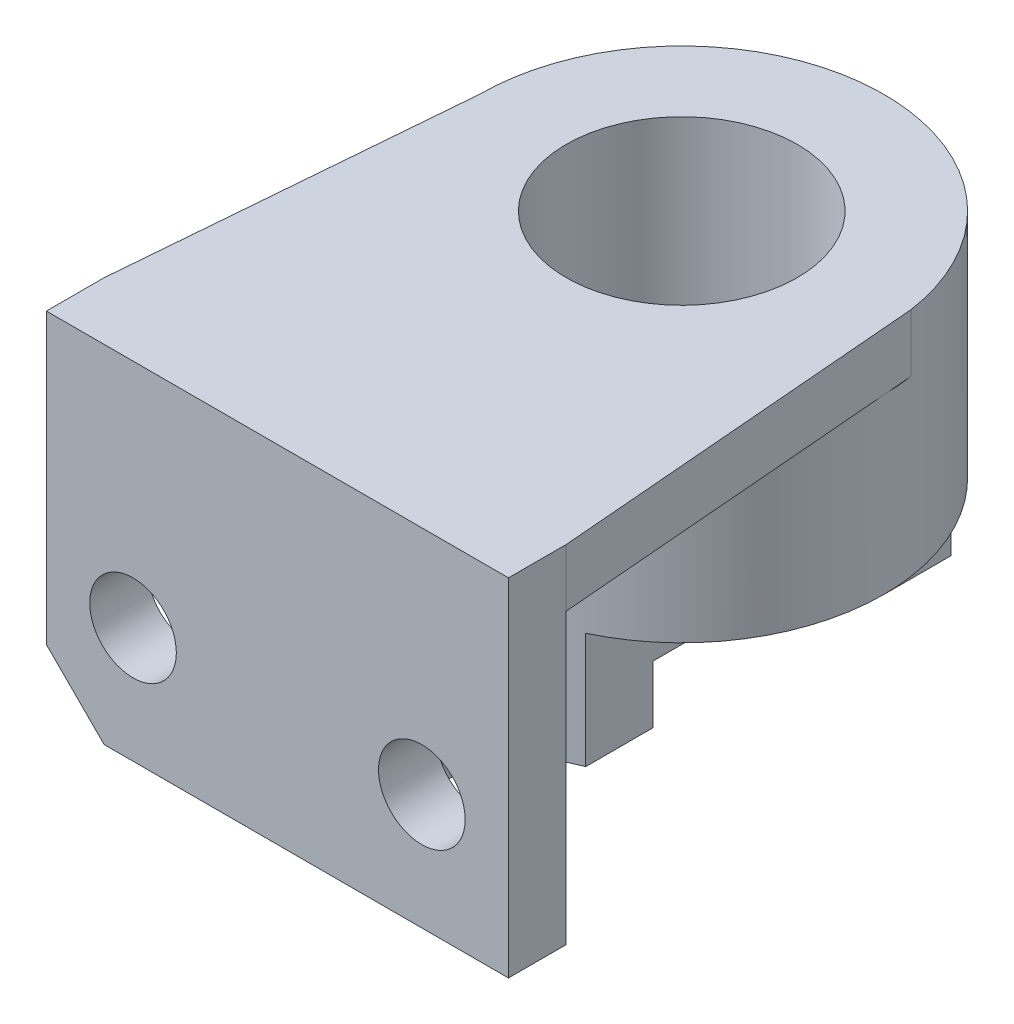
ISO-10303-21;
HEADER;
FILE_DESCRIPTION(('STEP AP214'),'2;1');
FILE_NAME('part.step','',(''),(''),'','','');
FILE_SCHEMA(('AUTOMOTIVE_DESIGN { 1 0 10303 214 1 1 1 1 }'));
ENDSEC;
DATA;
#1=APPLICATION_CONTEXT('core data for automotive mechanical design processes');
#2=APPLICATION_PROTOCOL_DEFINITION('international standard','automotive_design',2000,#1);
#3=PRODUCT_CONTEXT('',#1,'mechanical');
#4=PRODUCT('Part','Part','',(#3));
#5=PRODUCT_RELATED_PRODUCT_CATEGORY('part','',(#4));
#6=PRODUCT_DEFINITION_FORMATION('','',#4);
#7=PRODUCT_DEFINITION_CONTEXT('part definition',#1,'design');
#8=PRODUCT_DEFINITION('design','',#6,#7);
#9=PRODUCT_DEFINITION_SHAPE('','',#8);
#10=(LENGTH_UNIT() NAMED_UNIT(*) SI_UNIT(.MILLI.,.METRE.));
#11=(NAMED_UNIT(*) PLANE_ANGLE_UNIT() SI_UNIT($,.RADIAN.));
#12=(NAMED_UNIT(*) SI_UNIT($,.STERADIAN.) SOLID_ANGLE_UNIT());
#13=UNCERTAINTY_MEASURE_WITH_UNIT(LENGTH_MEASURE(1.E-05),#10,'distance_accuracy_value','');
#14=(GEOMETRIC_REPRESENTATION_CONTEXT(3) GLOBAL_UNCERTAINTY_ASSIGNED_CONTEXT((#13)) GLOBAL_UNIT_ASSIGNED_CONTEXT((#10,
#11,#12)) REPRESENTATION_CONTEXT('',''));
#15=CARTESIAN_POINT('',(0.,0.,0.));
#16=DIRECTION('',(0.,0.,1.));
#17=DIRECTION('',(1.,0.,0.));
#18=AXIS2_PLACEMENT_3D('',#15,#16,#17);
#19=CARTESIAN_POINT('',(40.,10.,-60.));
#20=DIRECTION('',(0.,-1.,0.));
#21=DIRECTION('',(0.,0.,-1.));
#22=AXIS2_PLACEMENT_3D('',#19,#20,#21);
#23=PLANE('',#22);
#24=CARTESIAN_POINT('',(40.,10.,-60.));
#25=DIRECTION('',(0.,-1.,0.));
#26=DIRECTION('',(0.,0.,-1.));
#27=AXIS2_PLACEMENT_3D('',#24,#25,#26);
#28=CIRCLE('',#27,20.);
#29=CARTESIAN_POINT('',(55.,10.,-73.228756555323));
#30=VERTEX_POINT('',#29);
#31=CARTESIAN_POINT('',(55.,10.,-46.771243444677));
#32=VERTEX_POINT('',#31);
#33=EDGE_CURVE('E213',#30,#32,#28,.T.);
#34=ORIENTED_EDGE('',*,*,#33,.F.);
#35=DIRECTION('',(0.,0.,-1.));
#36=VECTOR('',#35,1.);
#37=CARTESIAN_POINT('',(55.,10.,-28.3772233983162));
#38=LINE('',#37,#36);
#39=CARTESIAN_POINT('',(55.,10.,-91.6227766016838));
#40=VERTEX_POINT('',#39);
#41=EDGE_CURVE('E212',#30,#40,#38,.T.);
#42=ORIENTED_EDGE('',*,*,#41,.T.);
#43=CARTESIAN_POINT('',(40.,10.,-60.));
#44=DIRECTION('',(0.,-1.,0.));
#45=DIRECTION('',(0.,0.,-1.));
#46=AXIS2_PLACEMENT_3D('',#43,#44,#45);
#47=CIRCLE('',#46,35.);
#48=CARTESIAN_POINT('',(55.,10.,-28.3772233983162));
#49=VERTEX_POINT('',#48);
#50=EDGE_CURVE('E230',#40,#49,#47,.T.);
#51=ORIENTED_EDGE('',*,*,#50,.T.);
#52=EDGE_CURVE('E217',#49,#32,#38,.T.);
#53=ORIENTED_EDGE('',*,*,#52,.T.);
#54=EDGE_LOOP('',(#34,#42,#51,#53));
#55=FACE_BOUND('',#54,.T.);
#56=ADVANCED_FACE('F50',(#55),#23,.T.);
#57=CARTESIAN_POINT('',(40.,-10.,-60.));
#58=DIRECTION('',(0.,-1.,0.));
#59=DIRECTION('',(0.,0.,-1.));
#60=AXIS2_PLACEMENT_3D('',#57,#58,#59);
#61=PLANE('',#60);
#62=DIRECTION('',(0.,0.,-1.));
#63=VECTOR('',#62,1.);
#64=CARTESIAN_POINT('',(55.,-10.,-28.3772233983162));
#65=LINE('',#64,#63);
#66=CARTESIAN_POINT('',(55.,-10.,-28.3772233983162));
#67=VERTEX_POINT('',#66);
#68=CARTESIAN_POINT('',(55.,-10.,-40.));
#69=VERTEX_POINT('',#68);
#70=EDGE_CURVE('E445',#67,#69,#65,.T.);
#71=ORIENTED_EDGE('',*,*,#70,.F.);
#72=CARTESIAN_POINT('',(40.,-10.,-60.));
#73=DIRECTION('',(0.,-1.,0.));
#74=DIRECTION('',(0.,0.,-1.));
#75=AXIS2_PLACEMENT_3D('',#72,#73,#74);
#76=CIRCLE('',#75,35.);
#77=CARTESIAN_POINT('',(45.0000000000001,-10.,-25.3589838486225));
#78=VERTEX_POINT('',#77);
#79=EDGE_CURVE('E311',#67,#78,#76,.T.);
#80=ORIENTED_EDGE('',*,*,#79,.T.);
#81=DIRECTION('',(0.,0.,1.));
#82=VECTOR('',#81,1.);
#83=CARTESIAN_POINT('',(45.0000000000001,-10.,-25.3589838486225));
#84=LINE('',#83,#82);
#85=CARTESIAN_POINT('',(45.,-10.,0.));
#86=VERTEX_POINT('',#85);
#87=EDGE_CURVE('E288',#78,#86,#84,.T.);
#88=ORIENTED_EDGE('',*,*,#87,.T.);
#89=DIRECTION('',(1.,0.,0.));
#90=VECTOR('',#89,1.);
#91=CARTESIAN_POINT('',(0.,-10.,0.));
#92=LINE('',#91,#90);
#93=CARTESIAN_POINT('',(80.,-10.,0.));
#94=VERTEX_POINT('',#93);
#95=EDGE_CURVE('E282',#86,#94,#92,.T.);
#96=ORIENTED_EDGE('',*,*,#95,.T.);
#97=DIRECTION('',(0.,0.,1.));
#98=VECTOR('',#97,1.);
#99=CARTESIAN_POINT('',(80.,-10.,0.));
#100=LINE('',#99,#98);
#101=CARTESIAN_POINT('',(80.,-10.,10.));
#102=VERTEX_POINT('',#101);
#103=EDGE_CURVE('E276',#94,#102,#100,.T.);
#104=ORIENTED_EDGE('',*,*,#103,.T.);
#105=DIRECTION('',(1.,0.,0.));
#106=VECTOR('',#105,1.);
#107=CARTESIAN_POINT('',(0.,-10.,10.));
#108=LINE('',#107,#106);
#109=CARTESIAN_POINT('',(10.,-10.,10.));
#110=VERTEX_POINT('',#109);
#111=EDGE_CURVE('E278',#110,#102,#108,.T.);
#112=ORIENTED_EDGE('',*,*,#111,.F.);
#113=DIRECTION('',(0.,0.,1.));
#114=VECTOR('',#113,1.);
#115=CARTESIAN_POINT('',(10.,-10.,0.));
#116=LINE('',#115,#114);
#117=CARTESIAN_POINT('',(9.99999999999999,-10.,0.));
#118=VERTEX_POINT('',#117);
#119=EDGE_CURVE('E272',#118,#110,#116,.T.);
#120=ORIENTED_EDGE('',*,*,#119,.F.);
#121=CARTESIAN_POINT('',(35.,-10.,0.));
#122=VERTEX_POINT('',#121);
#123=EDGE_CURVE('E277',#118,#122,#92,.T.);
#124=ORIENTED_EDGE('',*,*,#123,.T.);
#125=DIRECTION('',(0.,0.,-1.));
#126=VECTOR('',#125,1.);
#127=CARTESIAN_POINT('',(35.,-10.,0.));
#128=LINE('',#127,#126);
#129=CARTESIAN_POINT('',(35.,-10.,-25.3589838486225));
#130=VERTEX_POINT('',#129);
#131=EDGE_CURVE('E283',#122,#130,#128,.T.);
#132=ORIENTED_EDGE('',*,*,#131,.T.);
#133=CARTESIAN_POINT('',(25.,-10.,-28.3772233983162));
#134=VERTEX_POINT('',#133);
#135=EDGE_CURVE('E306',#130,#134,#76,.T.);
#136=ORIENTED_EDGE('',*,*,#135,.T.);
#137=DIRECTION('',(0.,0.,1.));
#138=VECTOR('',#137,1.);
#139=CARTESIAN_POINT('',(25.,-10.,-91.6227766016838));
#140=LINE('',#139,#138);
#141=CARTESIAN_POINT('',(25.,-10.,-40.));
#142=VERTEX_POINT('',#141);
#143=EDGE_CURVE('E426',#142,#134,#140,.T.);
#144=ORIENTED_EDGE('',*,*,#143,.F.);
#145=CARTESIAN_POINT('',(40.,-10.,-60.));
#146=DIRECTION('',(0.,-1.,0.));
#147=DIRECTION('',(0.,0.,-1.));
#148=AXIS2_PLACEMENT_3D('',#145,#146,#147);
#149=CIRCLE('',#148,25.);
#150=EDGE_CURVE('E254',#69,#142,#149,.T.);
#151=ORIENTED_EDGE('',*,*,#150,.F.);
#152=EDGE_LOOP('',(#71,#80,#88,#96,#104,#112,#120,#124,#132,#136,#144,#151));
#153=FACE_BOUND('',#152,.T.);
#154=ADVANCED_FACE('F397',(#153),#61,.T.);
#155=CARTESIAN_POINT('',(40.,0.,-60.));
#156=DIRECTION('',(0.,-1.,0.));
#157=DIRECTION('',(0.,0.,-1.));
#158=AXIS2_PLACEMENT_3D('',#155,#156,#157);
#159=CYLINDRICAL_SURFACE('',#158,25.);
#160=CARTESIAN_POINT('',(25.,-10.,-80.));
#161=VERTEX_POINT('',#160);
#162=CARTESIAN_POINT('',(55.,-10.,-80.));
#163=VERTEX_POINT('',#162);
#164=EDGE_CURVE('E251',#161,#163,#149,.T.);
#165=ORIENTED_EDGE('',*,*,#164,.T.);
#166=DIRECTION('',(0.,-1.,0.));
#167=VECTOR('',#166,1.);
#168=CARTESIAN_POINT('',(55.,0.,-80.));
#169=LINE('',#168,#167);
#170=CARTESIAN_POINT('',(55.,0.,-80.));
#171=VERTEX_POINT('',#170);
#172=EDGE_CURVE('E237',#163,#171,#169,.F.);
#173=ORIENTED_EDGE('',*,*,#172,.T.);
#174=CARTESIAN_POINT('',(40.,0.,-60.));
#175=DIRECTION('',(0.,-1.,0.));
#176=DIRECTION('',(0.,0.,-1.));
#177=AXIS2_PLACEMENT_3D('',#174,#175,#176);
#178=CIRCLE('',#177,25.);
#179=CARTESIAN_POINT('',(25.,0.,-80.));
#180=VERTEX_POINT('',#179);
#181=EDGE_CURVE('E248',#180,#171,#178,.T.);
#182=ORIENTED_EDGE('',*,*,#181,.F.);
#183=DIRECTION('',(0.,-1.,0.));
#184=VECTOR('',#183,1.);
#185=CARTESIAN_POINT('',(25.,0.,-80.));
#186=LINE('',#185,#184);
#187=EDGE_CURVE('E451',#180,#161,#186,.T.);
#188=ORIENTED_EDGE('',*,*,#187,.T.);
#189=EDGE_LOOP('',(#165,#173,#182,#188));
#190=FACE_BOUND('',#189,.T.);
#191=ADVANCED_FACE('F496',(#190),#159,.F.);
#192=CARTESIAN_POINT('',(40.,0.,-60.));
#193=DIRECTION('',(0.,-1.,0.));
#194=DIRECTION('',(0.,0.,-1.));
#195=AXIS2_PLACEMENT_3D('',#192,#193,#194);
#196=PLANE('',#195);
#197=DIRECTION('',(0.,0.,-1.));
#198=VECTOR('',#197,1.);
#199=CARTESIAN_POINT('',(55.,0.,-60.));
#200=LINE('',#199,#198);
#201=CARTESIAN_POINT('',(55.,0.,-40.));
#202=VERTEX_POINT('',#201);
#203=CARTESIAN_POINT('',(55.,0.,-46.771243444677));
#204=VERTEX_POINT('',#203);
#205=EDGE_CURVE('E241',#202,#204,#200,.T.);
#206=ORIENTED_EDGE('',*,*,#205,.F.);
#207=CARTESIAN_POINT('',(25.,0.,-40.));
#208=VERTEX_POINT('',#207);
#209=EDGE_CURVE('E255',#202,#208,#178,.T.);
#210=ORIENTED_EDGE('',*,*,#209,.T.);
#211=DIRECTION('',(0.,0.,1.));
#212=VECTOR('',#211,1.);
#213=CARTESIAN_POINT('',(25.,0.,-60.));
#214=LINE('',#213,#212);
#215=CARTESIAN_POINT('',(25.,0.,-46.7712434446771));
#216=VERTEX_POINT('',#215);
#217=EDGE_CURVE('E454',#216,#208,#214,.T.);
#218=ORIENTED_EDGE('',*,*,#217,.F.);
#219=CARTESIAN_POINT('',(40.,0.,-60.));
#220=DIRECTION('',(0.,-1.,0.));
#221=DIRECTION('',(0.,0.,-1.));
#222=AXIS2_PLACEMENT_3D('',#219,#220,#221);
#223=CIRCLE('',#222,20.);
#224=EDGE_CURVE('E247',#204,#216,#223,.T.);
#225=ORIENTED_EDGE('',*,*,#224,.F.);
#226=EDGE_LOOP('',(#206,#210,#218,#225));
#227=FACE_BOUND('',#226,.T.);
#228=ADVANCED_FACE('F444',(#227),#196,.T.);
#229=CARTESIAN_POINT('',(0.,0.,0.));
#230=DIRECTION('',(0.,0.,1.));
#231=DIRECTION('',(1.,0.,0.));
#232=AXIS2_PLACEMENT_3D('',#229,#230,#231);
#233=PLANE('',#232);
#234=CARTESIAN_POINT('',(65.,10.,0.));
#235=DIRECTION('',(0.,0.,1.));
#236=DIRECTION('',(1.,0.,0.));
#237=AXIS2_PLACEMENT_3D('',#234,#235,#236);
#238=CIRCLE('',#237,7.50000000000001);
#239=CARTESIAN_POINT('',(72.5,10.,0.));
#240=VERTEX_POINT('',#239);
#241=EDGE_CURVE('E261',#240,#240,#238,.T.);
#242=ORIENTED_EDGE('',*,*,#241,.T.);
#243=EDGE_LOOP('',(#242));
#244=FACE_BOUND('',#243,.T.);
#245=DIRECTION('',(0.,1.,0.));
#246=VECTOR('',#245,1.);
#247=CARTESIAN_POINT('',(80.,10.,0.));
#248=LINE('',#247,#246);
#249=CARTESIAN_POINT('',(80.,40.,0.));
#250=VERTEX_POINT('',#249);
#251=EDGE_CURVE('E345',#94,#250,#248,.T.);
#252=ORIENTED_EDGE('',*,*,#251,.F.);
#253=ORIENTED_EDGE('',*,*,#95,.F.);
#254=DIRECTION('',(0.,-1.,0.));
#255=VECTOR('',#254,1.);
#256=CARTESIAN_POINT('',(45.,40.,0.));
#257=LINE('',#256,#255);
#258=CARTESIAN_POINT('',(45.,40.,0.));
#259=VERTEX_POINT('',#258);
#260=EDGE_CURVE('E294',#259,#86,#257,.T.);
#261=ORIENTED_EDGE('',*,*,#260,.F.);
#262=DIRECTION('',(-1.,0.,0.));
#263=VECTOR('',#262,1.);
#264=CARTESIAN_POINT('',(0.,40.,0.));
#265=LINE('',#264,#263);
#266=EDGE_CURVE('E324',#250,#259,#265,.T.);
#267=ORIENTED_EDGE('',*,*,#266,.F.);
#268=EDGE_LOOP('',(#252,#253,#261,#267));
#269=FACE_BOUND('',#268,.T.);
#270=ADVANCED_FACE('F401',(#244,#269),#233,.F.);
#271=CARTESIAN_POINT('',(0.,40.,0.));
#272=DIRECTION('',(0.,1.,0.));
#273=DIRECTION('',(0.,0.,1.));
#274=AXIS2_PLACEMENT_3D('',#271,#272,#273);
#275=PLANE('',#274);
#276=ORIENTED_EDGE('',*,*,#266,.T.);
#277=DIRECTION('',(0.,0.,1.));
#278=VECTOR('',#277,1.);
#279=CARTESIAN_POINT('',(45.0000000000001,40.,-25.3589838486225));
#280=LINE('',#279,#278);
#281=CARTESIAN_POINT('',(45.0000000000001,40.,-25.3589838486225));
#282=VERTEX_POINT('',#281);
#283=EDGE_CURVE('E290',#282,#259,#280,.T.);
#284=ORIENTED_EDGE('',*,*,#283,.F.);
#285=CARTESIAN_POINT('',(40.,40.,-60.));
#286=DIRECTION('',(0.,1.,0.));
#287=DIRECTION('',(0.,0.,1.));
#288=AXIS2_PLACEMENT_3D('',#285,#286,#287);
#289=CIRCLE('',#288,35.);
#290=CARTESIAN_POINT('',(74.9933136553649,40.,-60.6841048291398));
#291=VERTEX_POINT('',#290);
#292=EDGE_CURVE('E11',#291,#282,#289,.F.);
#293=ORIENTED_EDGE('',*,*,#292,.F.);
#294=DIRECTION('',(-0.0822247076971217,0.,-0.996613815599665));
#295=VECTOR('',#294,1.);
#296=CARTESIAN_POINT('',(79.4591277955298,40.,-6.55570237396765));
#297=LINE('',#296,#295);
#298=EDGE_CURVE('E313',#250,#291,#297,.T.);
#299=ORIENTED_EDGE('',*,*,#298,.F.);
#300=EDGE_LOOP('',(#276,#284,#293,#299));
#301=FACE_BOUND('',#300,.T.);
#302=ADVANCED_FACE('F390',(#301),#275,.F.);
#303=CARTESIAN_POINT('',(15.,10.,0.));
#304=DIRECTION('',(0.,0.,1.));
#305=DIRECTION('',(1.,0.,0.));
#306=AXIS2_PLACEMENT_3D('',#303,#304,#305);
#307=CIRCLE('',#306,7.5);
#308=CARTESIAN_POINT('',(22.5,10.,0.));
#309=VERTEX_POINT('',#308);
#310=EDGE_CURVE('E259',#309,#309,#307,.T.);
#311=ORIENTED_EDGE('',*,*,#310,.T.);
#312=EDGE_LOOP('',(#311));
#313=FACE_BOUND('',#312,.T.);
#314=ORIENTED_EDGE('',*,*,#123,.F.);
#315=DIRECTION('',(-0.707106781186548,0.707106781186548,0.));
#316=VECTOR('',#315,1.);
#317=CARTESIAN_POINT('',(10.,-10.,0.));
#318=LINE('',#317,#316);
#319=CARTESIAN_POINT('',(0.,0.,0.));
#320=VERTEX_POINT('',#319);
#321=EDGE_CURVE('E68',#118,#320,#318,.T.);
#322=ORIENTED_EDGE('',*,*,#321,.T.);
#323=DIRECTION('',(0.,-1.,0.));
#324=VECTOR('',#323,1.);
#325=CARTESIAN_POINT('',(0.,50.,0.));
#326=LINE('',#325,#324);
#327=CARTESIAN_POINT('',(0.,40.,0.));
#328=VERTEX_POINT('',#327);
#329=EDGE_CURVE('E337',#328,#320,#326,.T.);
#330=ORIENTED_EDGE('',*,*,#329,.F.);
#331=CARTESIAN_POINT('',(35.,40.,0.));
#332=VERTEX_POINT('',#331);
#333=EDGE_CURVE('E323',#332,#328,#265,.T.);
#334=ORIENTED_EDGE('',*,*,#333,.F.);
#335=DIRECTION('',(0.,-1.,0.));
#336=VECTOR('',#335,1.);
#337=CARTESIAN_POINT('',(35.,40.,0.));
#338=LINE('',#337,#336);
#339=EDGE_CURVE('E293',#332,#122,#338,.T.);
#340=ORIENTED_EDGE('',*,*,#339,.T.);
#341=EDGE_LOOP('',(#314,#322,#330,#334,#340));
#342=FACE_BOUND('',#341,.T.);
#343=ADVANCED_FACE('F420',(#313,#342),#233,.F.);
#344=CARTESIAN_POINT('',(0.,50.,10.));
#345=DIRECTION('',(1.,0.,0.));
#346=DIRECTION('',(0.,0.,-1.));
#347=AXIS2_PLACEMENT_3D('',#344,#345,#346);
#348=PLANE('',#347);
#349=ORIENTED_EDGE('',*,*,#329,.T.);
#350=DIRECTION('',(0.,0.,1.));
#351=VECTOR('',#350,1.);
#352=CARTESIAN_POINT('',(0.,0.,0.));
#353=LINE('',#352,#351);
#354=CARTESIAN_POINT('',(0.,0.,10.));
#355=VERTEX_POINT('',#354);
#356=EDGE_CURVE('E271',#320,#355,#353,.T.);
#357=ORIENTED_EDGE('',*,*,#356,.T.);
#358=DIRECTION('',(0.,-1.,0.));
#359=VECTOR('',#358,1.);
#360=CARTESIAN_POINT('',(0.,50.,10.));
#361=LINE('',#360,#359);
#362=CARTESIAN_POINT('',(0.,50.,10.));
#363=VERTEX_POINT('',#362);
#364=EDGE_CURVE('E338',#363,#355,#361,.T.);
#365=ORIENTED_EDGE('',*,*,#364,.F.);
#366=DIRECTION('',(0.,0.,-1.));
#367=VECTOR('',#366,1.);
#368=CARTESIAN_POINT('',(0.,50.,10.));
#369=LINE('',#368,#367);
#370=CARTESIAN_POINT('',(0.,50.,0.));
#371=VERTEX_POINT('',#370);
#372=EDGE_CURVE('E349',#363,#371,#369,.T.);
#373=ORIENTED_EDGE('',*,*,#372,.T.);
#374=EDGE_CURVE('E346',#371,#328,#326,.T.);
#375=ORIENTED_EDGE('',*,*,#374,.T.);
#376=EDGE_LOOP('',(#349,#357,#365,#373,#375));
#377=FACE_BOUND('',#376,.T.);
#378=ADVANCED_FACE('F47',(#377),#348,.F.);
#379=CARTESIAN_POINT('',(80.,10.,10.));
#380=DIRECTION('',(-1.,0.,0.));
#381=DIRECTION('',(0.,0.,1.));
#382=AXIS2_PLACEMENT_3D('',#379,#380,#381);
#383=PLANE('',#382);
#384=ORIENTED_EDGE('',*,*,#251,.T.);
#385=DIRECTION('',(0.,1.,0.));
#386=VECTOR('',#385,1.);
#387=CARTESIAN_POINT('',(80.,40.,0.));
#388=LINE('',#387,#386);
#389=CARTESIAN_POINT('',(80.,50.,0.));
#390=VERTEX_POINT('',#389);
#391=EDGE_CURVE('E333',#250,#390,#388,.T.);
#392=ORIENTED_EDGE('',*,*,#391,.T.);
#393=DIRECTION('',(0.,0.,-1.));
#394=VECTOR('',#393,1.);
#395=CARTESIAN_POINT('',(80.,50.,10.));
#396=LINE('',#395,#394);
#397=CARTESIAN_POINT('',(80.,50.,10.));
#398=VERTEX_POINT('',#397);
#399=EDGE_CURVE('E353',#398,#390,#396,.T.);
#400=ORIENTED_EDGE('',*,*,#399,.F.);
#401=DIRECTION('',(0.,1.,0.));
#402=VECTOR('',#401,1.);
#403=CARTESIAN_POINT('',(80.,10.,10.));
#404=LINE('',#403,#402);
#405=EDGE_CURVE('E342',#102,#398,#404,.T.);
#406=ORIENTED_EDGE('',*,*,#405,.F.);
#407=ORIENTED_EDGE('',*,*,#103,.F.);
#408=EDGE_LOOP('',(#384,#392,#400,#406,#407));
#409=FACE_BOUND('',#408,.T.);
#410=ADVANCED_FACE('F403',(#409),#383,.F.);
#411=CARTESIAN_POINT('',(80.,50.,10.));
#412=DIRECTION('',(0.,-1.,0.));
#413=DIRECTION('',(0.,0.,-1.));
#414=AXIS2_PLACEMENT_3D('',#411,#412,#413);
#415=PLANE('',#414);
#416=CARTESIAN_POINT('',(40.,50.,-60.));
#417=DIRECTION('',(0.,-1.,0.));
#418=DIRECTION('',(0.,0.,-1.));
#419=AXIS2_PLACEMENT_3D('',#416,#417,#418);
#420=CIRCLE('',#419,20.);
#421=CARTESIAN_POINT('',(40.,50.,-80.));
#422=VERTEX_POINT('',#421);
#423=EDGE_CURVE('E218',#422,#422,#420,.T.);
#424=ORIENTED_EDGE('',*,*,#423,.T.);
#425=EDGE_LOOP('',(#424));
#426=FACE_BOUND('',#425,.T.);
#427=ORIENTED_EDGE('',*,*,#399,.T.);
#428=DIRECTION('',(-0.0822247076971217,0.,-0.996613815599665));
#429=VECTOR('',#428,1.);
#430=CARTESIAN_POINT('',(79.4591277955298,50.,-6.55570237396765));
#431=LINE('',#430,#429);
#432=CARTESIAN_POINT('',(74.6322605792134,50.,-65.0602892381227));
#433=VERTEX_POINT('',#432);
#434=EDGE_CURVE('E307',#390,#433,#431,.T.);
#435=ORIENTED_EDGE('',*,*,#434,.T.);
#436=CARTESIAN_POINT('',(40.,50.,-60.));
#437=DIRECTION('',(0.,1.,0.));
#438=DIRECTION('',(0.,0.,1.));
#439=AXIS2_PLACEMENT_3D('',#436,#437,#438);
#440=CIRCLE('',#439,35.);
#441=CARTESIAN_POINT('',(4.99999999999999,50.,-60.));
#442=VERTEX_POINT('',#441);
#443=EDGE_CURVE('E329',#433,#442,#440,.T.);
#444=ORIENTED_EDGE('',*,*,#443,.T.);
#445=DIRECTION('',(-0.0830454798537398,0.,0.99654575824488));
#446=VECTOR('',#445,1.);
#447=CARTESIAN_POINT('',(0.,50.,0.));
#448=LINE('',#447,#446);
#449=EDGE_CURVE('E334',#442,#371,#448,.T.);
#450=ORIENTED_EDGE('',*,*,#449,.T.);
#451=ORIENTED_EDGE('',*,*,#372,.F.);
#452=DIRECTION('',(-1.,0.,0.));
#453=VECTOR('',#452,1.);
#454=CARTESIAN_POINT('',(80.,50.,10.));
#455=LINE('',#454,#453);
#456=EDGE_CURVE('E347',#398,#363,#455,.T.);
#457=ORIENTED_EDGE('',*,*,#456,.F.);
#458=EDGE_LOOP('',(#427,#435,#444,#450,#451,#457));
#459=FACE_BOUND('',#458,.T.);
#460=ADVANCED_FACE('F377',(#426,#459),#415,.F.);
#461=CARTESIAN_POINT('',(0.,0.,10.));
#462=DIRECTION('',(0.,0.,1.));
#463=DIRECTION('',(1.,0.,0.));
#464=AXIS2_PLACEMENT_3D('',#461,#462,#463);
#465=PLANE('',#464);
#466=CARTESIAN_POINT('',(15.,10.,10.));
#467=DIRECTION('',(0.,0.,1.));
#468=DIRECTION('',(1.,0.,0.));
#469=AXIS2_PLACEMENT_3D('',#466,#467,#468);
#470=CIRCLE('',#469,7.5);
#471=CARTESIAN_POINT('',(22.5,10.,10.));
#472=VERTEX_POINT('',#471);
#473=EDGE_CURVE('E262',#472,#472,#470,.T.);
#474=ORIENTED_EDGE('',*,*,#473,.F.);
#475=EDGE_LOOP('',(#474));
#476=FACE_BOUND('',#475,.T.);
#477=CARTESIAN_POINT('',(65.,10.,10.));
#478=DIRECTION('',(0.,0.,1.));
#479=DIRECTION('',(1.,0.,0.));
#480=AXIS2_PLACEMENT_3D('',#477,#478,#479);
#481=CIRCLE('',#480,7.50000000000001);
#482=CARTESIAN_POINT('',(72.5,10.,10.));
#483=VERTEX_POINT('',#482);
#484=EDGE_CURVE('E266',#483,#483,#481,.T.);
#485=ORIENTED_EDGE('',*,*,#484,.F.);
#486=EDGE_LOOP('',(#485));
#487=FACE_BOUND('',#486,.T.);
#488=DIRECTION('',(-0.707106781186548,0.707106781186548,0.));
#489=VECTOR('',#488,1.);
#490=CARTESIAN_POINT('',(10.,-10.,10.));
#491=LINE('',#490,#489);
#492=EDGE_CURVE('E256',#110,#355,#491,.T.);
#493=ORIENTED_EDGE('',*,*,#492,.F.);
#494=ORIENTED_EDGE('',*,*,#111,.T.);
#495=ORIENTED_EDGE('',*,*,#405,.T.);
#496=ORIENTED_EDGE('',*,*,#456,.T.);
#497=ORIENTED_EDGE('',*,*,#364,.T.);
#498=EDGE_LOOP('',(#493,#494,#495,#496,#497));
#499=FACE_BOUND('',#498,.T.);
#500=ADVANCED_FACE('F412',(#476,#487,#499),#465,.T.);
#501=CARTESIAN_POINT('',(79.4591277955298,40.,-6.55570237396765));
#502=DIRECTION('',(0.996613815599665,0.,-0.0822247076971218));
#503=DIRECTION('',(-0.0822247076971218,0.,-0.996613815599665));
#504=AXIS2_PLACEMENT_3D('',#501,#502,#503);
#505=PLANE('',#504);
#506=ORIENTED_EDGE('',*,*,#434,.F.);
#507=ORIENTED_EDGE('',*,*,#391,.F.);
#508=ORIENTED_EDGE('',*,*,#298,.T.);
#509=CARTESIAN_POINT('',(74.6322605792134,40.,-65.0602892381227));
#510=VERTEX_POINT('',#509);
#511=EDGE_CURVE('E319',#291,#510,#297,.T.);
#512=ORIENTED_EDGE('',*,*,#511,.T.);
#513=DIRECTION('',(0.,1.,0.));
#514=VECTOR('',#513,1.);
#515=CARTESIAN_POINT('',(74.6322605792134,40.,-65.0602892381227));
#516=LINE('',#515,#514);
#517=EDGE_CURVE('E321',#510,#433,#516,.T.);
#518=ORIENTED_EDGE('',*,*,#517,.T.);
#519=EDGE_LOOP('',(#506,#507,#508,#512,#518));
#520=FACE_BOUND('',#519,.T.);
#521=ADVANCED_FACE('F383',(#520),#505,.T.);
#522=CARTESIAN_POINT('',(0.,40.,0.));
#523=DIRECTION('',(-0.99654575824488,0.,-0.0830454798537398));
#524=DIRECTION('',(-0.0830454798537398,0.,0.99654575824488));
#525=AXIS2_PLACEMENT_3D('',#522,#523,#524);
#526=PLANE('',#525);
#527=ORIENTED_EDGE('',*,*,#449,.F.);
#528=DIRECTION('',(0.,1.,0.));
#529=VECTOR('',#528,1.);
#530=CARTESIAN_POINT('',(4.99999999999999,40.,-60.));
#531=LINE('',#530,#529);
#532=CARTESIAN_POINT('',(4.99999999999999,40.,-60.));
#533=VERTEX_POINT('',#532);
#534=EDGE_CURVE('E340',#533,#442,#531,.T.);
#535=ORIENTED_EDGE('',*,*,#534,.F.);
#536=DIRECTION('',(-0.0830454798537398,0.,0.99654575824488));
#537=VECTOR('',#536,1.);
#538=CARTESIAN_POINT('',(0.,40.,0.));
#539=LINE('',#538,#537);
#540=EDGE_CURVE('E320',#533,#328,#539,.T.);
#541=ORIENTED_EDGE('',*,*,#540,.T.);
#542=ORIENTED_EDGE('',*,*,#374,.F.);
#543=EDGE_LOOP('',(#527,#535,#541,#542));
#544=FACE_BOUND('',#543,.T.);
#545=ADVANCED_FACE('F376',(#544),#526,.T.);
#546=CARTESIAN_POINT('',(40.,40.,-60.));
#547=DIRECTION('',(0.,1.,0.));
#548=DIRECTION('',(0.,0.,1.));
#549=AXIS2_PLACEMENT_3D('',#546,#547,#548);
#550=CYLINDRICAL_SURFACE('',#549,35.);
#551=DIRECTION('',(0.,-1.,0.));
#552=VECTOR('',#551,1.);
#553=CARTESIAN_POINT('',(55.,10.,-28.3772233983162));
#554=LINE('',#553,#552);
#555=EDGE_CURVE('E473',#49,#67,#554,.T.);
#556=ORIENTED_EDGE('',*,*,#555,.F.);
#557=ORIENTED_EDGE('',*,*,#50,.F.);
#558=DIRECTION('',(0.,-1.,0.));
#559=VECTOR('',#558,1.);
#560=CARTESIAN_POINT('',(55.,10.,-91.6227766016838));
#561=LINE('',#560,#559);
#562=CARTESIAN_POINT('',(55.,-10.,-91.6227766016838));
#563=VERTEX_POINT('',#562);
#564=EDGE_CURVE('E227',#40,#563,#561,.T.);
#565=ORIENTED_EDGE('',*,*,#564,.T.);
#566=CARTESIAN_POINT('',(25.,-10.,-91.6227766016838));
#567=VERTEX_POINT('',#566);
#568=EDGE_CURVE('E309',#567,#563,#76,.T.);
#569=ORIENTED_EDGE('',*,*,#568,.F.);
#570=DIRECTION('',(0.,-1.,0.));
#571=VECTOR('',#570,1.);
#572=CARTESIAN_POINT('',(25.,10.,-91.6227766016838));
#573=LINE('',#572,#571);
#574=CARTESIAN_POINT('',(25.,10.,-91.6227766016838));
#575=VERTEX_POINT('',#574);
#576=EDGE_CURVE('E461',#575,#567,#573,.T.);
#577=ORIENTED_EDGE('',*,*,#576,.F.);
#578=CARTESIAN_POINT('',(40.,10.,-60.));
#579=DIRECTION('',(0.,-1.,0.));
#580=DIRECTION('',(0.,0.,-1.));
#581=AXIS2_PLACEMENT_3D('',#578,#579,#580);
#582=CIRCLE('',#581,35.);
#583=CARTESIAN_POINT('',(25.,10.,-28.3772233983162));
#584=VERTEX_POINT('',#583);
#585=EDGE_CURVE('E470',#584,#575,#582,.T.);
#586=ORIENTED_EDGE('',*,*,#585,.F.);
#587=DIRECTION('',(0.,-1.,0.));
#588=VECTOR('',#587,1.);
#589=CARTESIAN_POINT('',(25.,10.,-28.3772233983162));
#590=LINE('',#589,#588);
#591=EDGE_CURVE('E424',#584,#134,#590,.T.);
#592=ORIENTED_EDGE('',*,*,#591,.T.);
#593=ORIENTED_EDGE('',*,*,#135,.F.);
#594=DIRECTION('',(0.,-1.,0.));
#595=VECTOR('',#594,1.);
#596=CARTESIAN_POINT('',(35.,40.,-25.3589838486225));
#597=LINE('',#596,#595);
#598=CARTESIAN_POINT('',(35.,40.,-25.3589838486225));
#599=VERTEX_POINT('',#598);
#600=EDGE_CURVE('E301',#599,#130,#597,.T.);
#601=ORIENTED_EDGE('',*,*,#600,.F.);
#602=EDGE_CURVE('E54',#599,#533,#289,.F.);
#603=ORIENTED_EDGE('',*,*,#602,.T.);
#604=ORIENTED_EDGE('',*,*,#534,.T.);
#605=ORIENTED_EDGE('',*,*,#443,.F.);
#606=ORIENTED_EDGE('',*,*,#517,.F.);
#607=CARTESIAN_POINT('',(40.,40.,-60.));
#608=DIRECTION('',(0.,-1.,0.));
#609=DIRECTION('',(0.,0.,-1.));
#610=AXIS2_PLACEMENT_3D('',#607,#608,#609);
#611=CIRCLE('',#610,35.);
#612=EDGE_CURVE('E300',#510,#291,#611,.T.);
#613=ORIENTED_EDGE('',*,*,#612,.T.);
#614=ORIENTED_EDGE('',*,*,#292,.T.);
#615=DIRECTION('',(0.,-1.,0.));
#616=VECTOR('',#615,1.);
#617=CARTESIAN_POINT('',(45.0000000000001,40.,-25.3589838486225));
#618=LINE('',#617,#616);
#619=EDGE_CURVE('E296',#282,#78,#618,.T.);
#620=ORIENTED_EDGE('',*,*,#619,.T.);
#621=ORIENTED_EDGE('',*,*,#79,.F.);
#622=EDGE_LOOP('',(#556,#557,#565,#569,#577,#586,#592,#593,#601,#603,#604,#605,#606,#613,#614,
#620,#621));
#623=FACE_BOUND('',#622,.T.);
#624=ADVANCED_FACE('F362',(#623),#550,.T.);
#625=ORIENTED_EDGE('',*,*,#602,.F.);
#626=DIRECTION('',(0.,0.,-1.));
#627=VECTOR('',#626,1.);
#628=CARTESIAN_POINT('',(35.,40.,0.));
#629=LINE('',#628,#627);
#630=EDGE_CURVE('E289',#332,#599,#629,.T.);
#631=ORIENTED_EDGE('',*,*,#630,.F.);
#632=ORIENTED_EDGE('',*,*,#333,.T.);
#633=ORIENTED_EDGE('',*,*,#540,.F.);
#634=EDGE_LOOP('',(#625,#631,#632,#633));
#635=FACE_BOUND('',#634,.T.);
#636=ADVANCED_FACE('F375',(#635),#275,.F.);
#637=EDGE_CURVE('E462',#163,#563,#65,.T.);
#638=ORIENTED_EDGE('',*,*,#637,.F.);
#639=ORIENTED_EDGE('',*,*,#164,.F.);
#640=EDGE_CURVE('E431',#567,#161,#140,.T.);
#641=ORIENTED_EDGE('',*,*,#640,.F.);
#642=ORIENTED_EDGE('',*,*,#568,.T.);
#643=EDGE_LOOP('',(#638,#639,#641,#642));
#644=FACE_BOUND('',#643,.T.);
#645=ADVANCED_FACE('F498',(#644),#61,.T.);
#646=CARTESIAN_POINT('',(40.,40.,-60.));
#647=DIRECTION('',(0.,-1.,0.));
#648=DIRECTION('',(0.,0.,-1.));
#649=AXIS2_PLACEMENT_3D('',#646,#647,#648);
#650=PLANE('',#649);
#651=ORIENTED_EDGE('',*,*,#511,.F.);
#652=ORIENTED_EDGE('',*,*,#612,.F.);
#653=EDGE_LOOP('',(#651,#652));
#654=FACE_BOUND('',#653,.T.);
#655=ADVANCED_FACE('F381',(#654),#650,.F.);
#656=CARTESIAN_POINT('',(45.0000000000001,40.,-25.3589838486225));
#657=DIRECTION('',(1.,0.,0.));
#658=DIRECTION('',(0.,0.,-1.));
#659=AXIS2_PLACEMENT_3D('',#656,#657,#658);
#660=PLANE('',#659);
#661=ORIENTED_EDGE('',*,*,#87,.F.);
#662=ORIENTED_EDGE('',*,*,#619,.F.);
#663=ORIENTED_EDGE('',*,*,#283,.T.);
#664=ORIENTED_EDGE('',*,*,#260,.T.);
#665=EDGE_LOOP('',(#661,#662,#663,#664));
#666=FACE_BOUND('',#665,.T.);
#667=ADVANCED_FACE('F391',(#666),#660,.T.);
#668=CARTESIAN_POINT('',(35.,40.,0.));
#669=DIRECTION('',(-1.,0.,0.));
#670=DIRECTION('',(0.,0.,1.));
#671=AXIS2_PLACEMENT_3D('',#668,#669,#670);
#672=PLANE('',#671);
#673=ORIENTED_EDGE('',*,*,#131,.F.);
#674=ORIENTED_EDGE('',*,*,#339,.F.);
#675=ORIENTED_EDGE('',*,*,#630,.T.);
#676=ORIENTED_EDGE('',*,*,#600,.T.);
#677=EDGE_LOOP('',(#673,#674,#675,#676));
#678=FACE_BOUND('',#677,.T.);
#679=ADVANCED_FACE('F423',(#678),#672,.T.);
#680=CARTESIAN_POINT('',(10.,-10.,0.));
#681=DIRECTION('',(0.707106781186548,0.707106781186548,0.));
#682=DIRECTION('',(-0.707106781186548,0.707106781186548,0.));
#683=AXIS2_PLACEMENT_3D('',#680,#681,#682);
#684=PLANE('',#683);
#685=ORIENTED_EDGE('',*,*,#492,.T.);
#686=ORIENTED_EDGE('',*,*,#356,.F.);
#687=ORIENTED_EDGE('',*,*,#321,.F.);
#688=ORIENTED_EDGE('',*,*,#119,.T.);
#689=EDGE_LOOP('',(#685,#686,#687,#688));
#690=FACE_BOUND('',#689,.T.);
#691=ADVANCED_FACE('F414',(#690),#684,.F.);
#692=CARTESIAN_POINT('',(65.,10.,0.));
#693=DIRECTION('',(0.,0.,1.));
#694=DIRECTION('',(1.,0.,0.));
#695=AXIS2_PLACEMENT_3D('',#692,#693,#694);
#696=CYLINDRICAL_SURFACE('',#695,7.50000000000001);
#697=ORIENTED_EDGE('',*,*,#241,.F.);
#698=EDGE_LOOP('',(#697));
#699=FACE_BOUND('',#698,.T.);
#700=ORIENTED_EDGE('',*,*,#484,.T.);
#701=EDGE_LOOP('',(#700));
#702=FACE_BOUND('',#701,.T.);
#703=ADVANCED_FACE('F566',(#699,#702),#696,.F.);
#704=CARTESIAN_POINT('',(15.,10.,0.));
#705=DIRECTION('',(0.,0.,1.));
#706=DIRECTION('',(1.,0.,0.));
#707=AXIS2_PLACEMENT_3D('',#704,#705,#706);
#708=CYLINDRICAL_SURFACE('',#707,7.5);
#709=ORIENTED_EDGE('',*,*,#310,.F.);
#710=EDGE_LOOP('',(#709));
#711=FACE_BOUND('',#710,.T.);
#712=ORIENTED_EDGE('',*,*,#473,.T.);
#713=EDGE_LOOP('',(#712));
#714=FACE_BOUND('',#713,.T.);
#715=ADVANCED_FACE('F595',(#711,#714),#708,.F.);
#716=ORIENTED_EDGE('',*,*,#209,.F.);
#717=DIRECTION('',(0.,-1.,0.));
#718=VECTOR('',#717,1.);
#719=CARTESIAN_POINT('',(55.,0.,-40.));
#720=LINE('',#719,#718);
#721=EDGE_CURVE('E240',#202,#69,#720,.T.);
#722=ORIENTED_EDGE('',*,*,#721,.T.);
#723=ORIENTED_EDGE('',*,*,#150,.T.);
#724=DIRECTION('',(0.,-1.,0.));
#725=VECTOR('',#724,1.);
#726=CARTESIAN_POINT('',(25.,0.,-40.));
#727=LINE('',#726,#725);
#728=EDGE_CURVE('E440',#142,#208,#727,.F.);
#729=ORIENTED_EDGE('',*,*,#728,.T.);
#730=EDGE_LOOP('',(#716,#722,#723,#729));
#731=FACE_BOUND('',#730,.T.);
#732=ADVANCED_FACE('F436',(#731),#159,.F.);
#733=CARTESIAN_POINT('',(55.,0.,-73.228756555323));
#734=VERTEX_POINT('',#733);
#735=EDGE_CURVE('E236',#734,#171,#200,.T.);
#736=ORIENTED_EDGE('',*,*,#735,.F.);
#737=CARTESIAN_POINT('',(25.,0.,-73.2287565553229));
#738=VERTEX_POINT('',#737);
#739=EDGE_CURVE('E232',#738,#734,#223,.T.);
#740=ORIENTED_EDGE('',*,*,#739,.F.);
#741=EDGE_CURVE('E459',#180,#738,#214,.T.);
#742=ORIENTED_EDGE('',*,*,#741,.F.);
#743=ORIENTED_EDGE('',*,*,#181,.T.);
#744=EDGE_LOOP('',(#736,#740,#742,#743));
#745=FACE_BOUND('',#744,.T.);
#746=ADVANCED_FACE('F484',(#745),#196,.T.);
#747=CARTESIAN_POINT('',(40.,10.,-60.));
#748=DIRECTION('',(0.,-1.,0.));
#749=DIRECTION('',(0.,0.,-1.));
#750=AXIS2_PLACEMENT_3D('',#747,#748,#749);
#751=CYLINDRICAL_SURFACE('',#750,20.);
#752=DIRECTION('',(0.,-1.,0.));
#753=VECTOR('',#752,1.);
#754=CARTESIAN_POINT('',(25.,10.,-46.7712434446771));
#755=LINE('',#754,#753);
#756=CARTESIAN_POINT('',(25.,10.,-46.7712434446771));
#757=VERTEX_POINT('',#756);
#758=EDGE_CURVE('E452',#216,#757,#755,.F.);
#759=ORIENTED_EDGE('',*,*,#758,.T.);
#760=CARTESIAN_POINT('',(25.,10.,-73.2287565553229));
#761=VERTEX_POINT('',#760);
#762=EDGE_CURVE('E64',#757,#761,#28,.T.);
#763=ORIENTED_EDGE('',*,*,#762,.T.);
#764=DIRECTION('',(0.,-1.,0.));
#765=VECTOR('',#764,1.);
#766=CARTESIAN_POINT('',(25.,10.,-73.2287565553229));
#767=LINE('',#766,#765);
#768=EDGE_CURVE('E458',#761,#738,#767,.T.);
#769=ORIENTED_EDGE('',*,*,#768,.T.);
#770=ORIENTED_EDGE('',*,*,#739,.T.);
#771=DIRECTION('',(0.,-1.,0.));
#772=VECTOR('',#771,1.);
#773=CARTESIAN_POINT('',(55.,10.,-73.228756555323));
#774=LINE('',#773,#772);
#775=EDGE_CURVE('E223',#734,#30,#774,.F.);
#776=ORIENTED_EDGE('',*,*,#775,.T.);
#777=ORIENTED_EDGE('',*,*,#33,.T.);
#778=DIRECTION('',(0.,-1.,0.));
#779=VECTOR('',#778,1.);
#780=CARTESIAN_POINT('',(55.,10.,-46.771243444677));
#781=LINE('',#780,#779);
#782=EDGE_CURVE('E449',#32,#204,#781,.T.);
#783=ORIENTED_EDGE('',*,*,#782,.T.);
#784=ORIENTED_EDGE('',*,*,#224,.T.);
#785=EDGE_LOOP('',(#759,#763,#769,#770,#776,#777,#783,#784));
#786=FACE_BOUND('',#785,.T.);
#787=ORIENTED_EDGE('',*,*,#423,.F.);
#788=EDGE_LOOP('',(#787));
#789=FACE_BOUND('',#788,.T.);
#790=ADVANCED_FACE('F235',(#786,#789),#751,.F.);
#791=ORIENTED_EDGE('',*,*,#762,.F.);
#792=DIRECTION('',(0.,0.,1.));
#793=VECTOR('',#792,1.);
#794=CARTESIAN_POINT('',(25.,10.,-91.6227766016838));
#795=LINE('',#794,#793);
#796=EDGE_CURVE('E469',#757,#584,#795,.T.);
#797=ORIENTED_EDGE('',*,*,#796,.T.);
#798=ORIENTED_EDGE('',*,*,#585,.T.);
#799=EDGE_CURVE('E463',#575,#761,#795,.T.);
#800=ORIENTED_EDGE('',*,*,#799,.T.);
#801=EDGE_LOOP('',(#791,#797,#798,#800));
#802=FACE_BOUND('',#801,.T.);
#803=ADVANCED_FACE('F478',(#802),#23,.T.);
#804=CARTESIAN_POINT('',(25.,10.,-91.6227766016838));
#805=DIRECTION('',(1.,0.,0.));
#806=DIRECTION('',(0.,0.,-1.));
#807=AXIS2_PLACEMENT_3D('',#804,#805,#806);
#808=PLANE('',#807);
#809=ORIENTED_EDGE('',*,*,#143,.T.);
#810=ORIENTED_EDGE('',*,*,#591,.F.);
#811=ORIENTED_EDGE('',*,*,#796,.F.);
#812=ORIENTED_EDGE('',*,*,#758,.F.);
#813=ORIENTED_EDGE('',*,*,#217,.T.);
#814=ORIENTED_EDGE('',*,*,#728,.F.);
#815=EDGE_LOOP('',(#809,#810,#811,#812,#813,#814));
#816=FACE_BOUND('',#815,.T.);
#817=ADVANCED_FACE('F487',(#816),#808,.F.);
#818=ORIENTED_EDGE('',*,*,#741,.T.);
#819=ORIENTED_EDGE('',*,*,#768,.F.);
#820=ORIENTED_EDGE('',*,*,#799,.F.);
#821=ORIENTED_EDGE('',*,*,#576,.T.);
#822=ORIENTED_EDGE('',*,*,#640,.T.);
#823=ORIENTED_EDGE('',*,*,#187,.F.);
#824=EDGE_LOOP('',(#818,#819,#820,#821,#822,#823));
#825=FACE_BOUND('',#824,.T.);
#826=ADVANCED_FACE('F505',(#825),#808,.F.);
#827=CARTESIAN_POINT('',(55.,10.,-28.3772233983162));
#828=DIRECTION('',(-1.,0.,0.));
#829=DIRECTION('',(0.,0.,1.));
#830=AXIS2_PLACEMENT_3D('',#827,#828,#829);
#831=PLANE('',#830);
#832=ORIENTED_EDGE('',*,*,#637,.T.);
#833=ORIENTED_EDGE('',*,*,#564,.F.);
#834=ORIENTED_EDGE('',*,*,#41,.F.);
#835=ORIENTED_EDGE('',*,*,#775,.F.);
#836=ORIENTED_EDGE('',*,*,#735,.T.);
#837=ORIENTED_EDGE('',*,*,#172,.F.);
#838=EDGE_LOOP('',(#832,#833,#834,#835,#836,#837));
#839=FACE_BOUND('',#838,.T.);
#840=ADVANCED_FACE('F225',(#839),#831,.F.);
#841=ORIENTED_EDGE('',*,*,#205,.T.);
#842=ORIENTED_EDGE('',*,*,#782,.F.);
#843=ORIENTED_EDGE('',*,*,#52,.F.);
#844=ORIENTED_EDGE('',*,*,#555,.T.);
#845=ORIENTED_EDGE('',*,*,#70,.T.);
#846=ORIENTED_EDGE('',*,*,#721,.F.);
#847=EDGE_LOOP('',(#841,#842,#843,#844,#845,#846));
#848=FACE_BOUND('',#847,.T.);
#849=ADVANCED_FACE('F441',(#848),#831,.F.);
#850=CLOSED_SHELL('',(#56,#154,#191,#228,#270,#302,#343,#378,#410,#460,#500,#521,#545,#624,#636,
#645,#655,#667,#679,#691,#703,#715,#732,#746,#790,#803,#817,#826,#840,#849));
#851=MANIFOLD_SOLID_BREP('B2',#850);
#852=ADVANCED_BREP_SHAPE_REPRESENTATION('',(#18,#851),#14);
#853=SHAPE_DEFINITION_REPRESENTATION(#9,#852);
ENDSEC;
END-ISO-10303-21;
